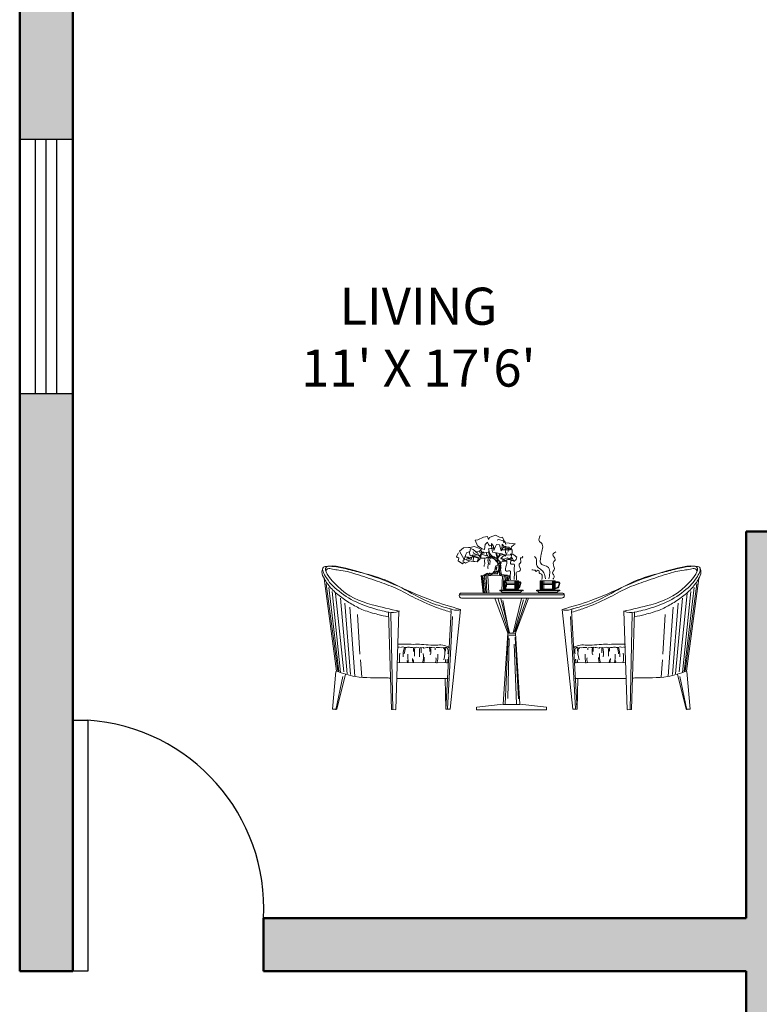
# Model space of a CAD drawing. Units: inches. Extents: x 1771 to 3025, y 319 to 889.
# Tile 2 of 35: x 1800 to 1939, y 527 to 713. Entities that reach past the tile are written whole.
import ezdxf

# ---------------------------------------------------------------- set-up
doc = ezdxf.new("R2010")
doc.units = ezdxf.units.IN
doc.header["$MEASUREMENT"] = 0
for name, color, linetype, lineweight in [('A-AREA-IDEN', 241, 'Continuous', 25), ('A-DOOR', 4, 'Continuous', 25), ('A-FURN', 8, 'Continuous', 18), ('A-GLAZ', 40, 'Continuous', 25), ('A-WALL', 7, 'Continuous', 50), ('A-WALL-PATT', 254, 'Continuous', 13)]:
    doc.layers.add(name, color=color, linetype=linetype, lineweight=lineweight)
doc.styles.get("Standard").update_dxf_attribs({"font": 'arial.ttf'})

# ---------------------------------------------------------------- blocks, each defined once
blk = doc.blocks.new('A$C7D4176DC')
for p, q in [((936.5, 1019.3), (919.6, 1018.3)), ((919.6, 1018.3), (933.7, 984.6)), ((969.3, 1036.1), (936.5, 1019.3)), ((994.5, 1040.8), (969.3, 1036.1)), ((980.5, 991.2), (994.5, 1005.2)), ((1000.2, 1022.1), (994.5, 1040.8)), ((994.5, 1005.2), (999.2, 992.1)), ((1008.6, 1036.1), (1000.2, 1022.1)), ((1010.5, 1037.1), (1041.4, 1048.3)), ((1041.4, 1048.3), (1064.8, 1036.1)), ((1051.7, 1018.3), (1059.2, 1023)), ((1059.2, 1023), (1090.1, 1013.6)), ((1064.8, 1036.1), (1077, 1034.2)), ((1077, 1034.2), (1084.5, 1035.2)), ((1084.5, 1035.2), (1097.6, 1007.1)), ((1091, 1009.9), (1088.2, 1005.2)), ((1088.2, 1005.2), (1104.1, 1009)), ((1090.1, 1013.6), (1091, 1009.9)), ((1104.1, 1009), (1091, 1005.2)), ((1091, 1005.2), (1100.4, 1003.4)), ((850.3, 971.5), (825.9, 951.9)), ((825.9, 951.9), (853.1, 902.3)), ((879.3, 973.4), (850.3, 971.5)), ((869, 944.4), (886.8, 949.1)), ((889.6, 974.3), (879.3, 973.4)), ((890.6, 924.7), (884, 950)), ((886.8, 949.1), (892.4, 968.7)), ((914, 980.9), (889.6, 974.3)), ((892.4, 968.7), (908.4, 962.2)), ((908.4, 962.2), (934.6, 940.6)), ((909.3, 940.6), (908.4, 947.2)), ((947.7, 967.8), (914, 980.9)), ((927.4, 947.9), (955.2, 956.5)), ((933.7, 984.6), (961.8, 966.8)), ((946.8, 953.7), (945.8, 946.2)), ((945.8, 946.2), (971.1, 945.3)), ((958, 965.9), (946.8, 953.7)), ((955.2, 956.5), (961.8, 934.1)), ((961.8, 966.8), (976.7, 961.2)), ((976.7, 961.2), (980.5, 991.2)), ((999.2, 992.1), (1006.7, 983.7)), ((999.2, 965.9), (1016.1, 967.8)), ((1003, 952.8), (999.2, 965.9)), ((999.2, 945.3), (1003, 952.8)), ((1002, 948.1), (1001.1, 940.6)), ((1012.3, 931.3), (1002, 948.1)), ((1006.7, 983.7), (1022.6, 987.4)), ((1022.6, 987.4), (1015.2, 989.3)), ((1016.1, 967.8), (1017, 970.6)), ((1029.2, 982.8), (1017, 998.7)), ((1017, 998.7), (1017, 981.8)), ((1017, 981.8), (1024.5, 946.2)), ((1017, 970.6), (1037.6, 969.7)), ((1024.5, 946.2), (1082.6, 936)), ((1032, 956.5), (1029.2, 982.8)), ((1042.3, 979.9), (1032, 956.5)), ((1037.6, 969.7), (1033, 971.5)), ((1047.9, 992.1), (1042.3, 979.9)), ((1066.7, 989.3), (1047.9, 992.1)), ((1075.1, 953.7), (1066.7, 989.3)), ((1079.8, 959.4), (1075.1, 953.7)), ((1081.7, 994), (1079.8, 959.4)), ((1095.7, 976.2), (1081.7, 994)), ((1103.2, 982.8), (1084.5, 969.7)), ((1084.5, 969.7), (1084.5, 959.4)), ((1084.5, 959.4), (1127.6, 960.3)), ((1121, 975.3), (1095.7, 976.2)), ((1100.4, 1003.4), (1103.2, 993.1)), ((1100.4, 971.5), (1103.2, 982.8)), ((1101.3, 940.6), (1100.4, 971.5)), ((1106, 966.8), (1104.1, 968.7)), ((1121, 969.7), (1106, 966.8)), ((1108.2, 1001.8), (1157.5, 996.8)), ((1119.1, 963.1), (1121, 969.7)), ((1127.6, 960.3), (1119.1, 963.1)), ((1132.2, 960.3), (1121, 975.3)), ((1137.9, 978.1), (1132.2, 960.3)), ((1151, 989.3), (1137.9, 978.1)), ((1159.4, 994), (1151, 989.3)), ((1157.5, 996.8), (1159.4, 994)), ((820.3, 941.6), (808.1, 920)), ((808.1, 920), (811.9, 913.5)), ((811.9, 913.5), (821.2, 911.6)), ((821.2, 911.6), (817.5, 893.8)), ((817.5, 893.8), (843.7, 875.1)), ((847.5, 897.6), (877.4, 906)), ((847.5, 880.7), (847.5, 897.6)), ((853.1, 902.3), (863.4, 931.3)), ((860.6, 917.2), (858.7, 916.3)), ((863.4, 917.2), (860.6, 917.2)), ((878.4, 916.3), (861.5, 919.1)), ((886.7, 892.7), (862.1, 880.4)), ((863.4, 931.3), (869, 944.4)), ((876.5, 911.6), (863.4, 917.2)), ((870.3, 898.8), (868.3, 907)), ((895, 892.7), (870.3, 898.8)), ((879.3, 906.9), (876.5, 911.6)), ((877.4, 906), (884.9, 905.1)), ((883.1, 912.5), (878.4, 916.3)), ((894.3, 912.5), (879.3, 906.9)), ((910.2, 917.2), (883.1, 912.5)), ((884.9, 905.1), (889.6, 903.2)), ((889.6, 903.2), (895.2, 901.3)), ((900.9, 928.5), (890.6, 924.7)), ((902.7, 916.3), (894.3, 912.5)), ((931.9, 888.6), (895, 892.7)), ((895.2, 901.3), (899, 917.2)), ((922.4, 927.5), (900.9, 928.5)), ((903.7, 927.5), (902.7, 916.3)), ((905.6, 928.5), (903.7, 927.5)), ((904.6, 923.8), (905.6, 928.5)), ((904.6, 920), (904.6, 923.8)), ((919.6, 920), (904.6, 920)), ((909.3, 913.2), (907.3, 892.7)), ((917.7, 936), (909.3, 940.6)), ((917.5, 890.6), (909.3, 890.6)), ((939.3, 910.7), (910.2, 917.2)), ((931.9, 888.6), (917.5, 890.6)), ((928, 933.1), (917.7, 936)), ((939.3, 913.5), (919.6, 920)), ((932.7, 929.4), (922.4, 927.5)), ((942.1, 925.7), (928, 933.1)), ((940.1, 909.1), (931.9, 888.6)), ((950.4, 907), (931.9, 888.6)), ((941.1, 929.4), (932.7, 929.4)), ((934.6, 940.6), (938.3, 938.8)), ((985.2, 912.5), (939.3, 910.7)), ((951.5, 911.6), (941.1, 929.4)), ((950.5, 917.2), (942.1, 925.7)), ((955.2, 940.6), (946.8, 924.7)), ((946.8, 924.7), (951.5, 918.2)), ((1026.4, 913.5), (950.4, 907.4)), ((952.4, 910.7), (950.5, 917.2)), ((959.9, 938.8), (951.5, 925.7)), ((951.5, 925.7), (954.3, 912.5)), ((951.5, 918.2), (951.5, 911.6)), ((954.3, 909.7), (955.2, 940.6)), ((954.3, 912.5), (954.3, 909.7)), ((986.1, 943.4), (960.8, 940.6)), ((961.8, 934.1), (984.2, 923.8)), ((967.4, 939.2), (999.2, 945.3)), ((976.2, 896.9), (974.8, 892)), ((974.8, 892), (977.6, 877.4)), ((978.3, 903.2), (976.2, 896.9)), ((977.6, 912.2), (978.3, 903.2)), ((984.2, 923.8), (995.5, 925.7)), ((988.9, 914.4), (985.2, 912.5)), ((989.9, 930.3), (986.1, 943.4)), ((991.7, 916.3), (988.9, 914.4)), ((989.5, 915.7), (998.5, 919.9)), ((995.5, 925.7), (989.9, 930.3)), ((1005.8, 917.2), (991.7, 916.3)), ((998.5, 904.6), (995.7, 898.3)), ((995.7, 898.3), (999.9, 878.8)), ((998.5, 919.9), (1000.6, 912.2)), ((1000.6, 912.2), (998.5, 904.6)), ((1001.1, 940.6), (1006.7, 926.6)), ((1006.9, 906), (1004.1, 898.3)), ((1004.1, 898.3), (1009, 894.8)), ((1007.7, 920), (1005.8, 917.2)), ((1006.7, 926.6), (1011.4, 921.9)), ((1011.8, 911.5), (1006.9, 906)), ((1006.9, 911.5), (1030.6, 908)), ((1009, 889.2), (1006.9, 877.4)), ((1027.3, 916.3), (1007.7, 920)), ((1009, 894.8), (1009, 889.2)), ((1009.7, 920.6), (1011.8, 911.5)), ((1011.4, 921.9), (1025.5, 914.4)), ((1021.7, 921.9), (1012.3, 931.3)), ((1033, 919.1), (1021.7, 921.9)), ((1025.5, 914.4), (1048.9, 908.8)), ((1030.6, 908), (1036.9, 901.1)), ((1046.7, 908.7), (1033, 919.1)), ((1036.9, 901.1), (1049.5, 899)), ((1039, 899), (1045.3, 891.3)), ((1049.5, 899), (1039, 899)), ((1047.9, 941.6), (1043.3, 939.7)), ((1043.3, 939.7), (1048.9, 920)), ((1045.3, 891.3), (1052.3, 886.4)), ((1055.4, 914.4), (1047.9, 941.6)), ((1048.9, 920), (1049.8, 910.7)), ((1048.9, 908.8), (1076, 881.7)), ((1049.8, 910.7), (1050.8, 902.3)), ((1050.8, 902.3), (1060.1, 872.3)), ((1058.2, 880.7), (1050.8, 894.8)), ((1067.6, 934.1), (1054.5, 910.7)), ((1054.5, 910.7), (1054.5, 898.5)), ((1054.5, 898.5), (1059.9, 896.9)), ((1056.4, 890.1), (1055.4, 914.4)), ((1056.4, 905.1), (1055.4, 895.7)), ((1055.4, 895.7), (1057.3, 892)), ((1061.1, 918.2), (1056.4, 905.1)), ((1064.8, 923.8), (1061.1, 918.2)), ((1067.6, 929.4), (1064.8, 927.5)), ((1066.7, 926.6), (1064.8, 923.8)), ((1089.2, 931.3), (1066.7, 926.6)), ((1084.5, 932.2), (1067.6, 929.4)), ((1070.4, 862.9), (1067.6, 890.1)), ((1072.3, 910), (1078.2, 913)), ((1091.3, 904.2), (1072.3, 910)), ((1097.2, 895.4), (1076.7, 886.6)), ((1078.2, 913), (1100.1, 932)), ((1082.6, 936), (1096.7, 928.5)), ((1098.6, 893.9), (1089.9, 904.2)), ((1113.3, 911.5), (1091.3, 904.2)), ((1096.7, 928.5), (1101.3, 922.8)), ((1100.1, 932), (1097.2, 927.6)), ((1097.2, 927.6), (1117.7, 930.5)), ((1113.3, 902.7), (1097.2, 895.4)), ((1113.3, 899.8), (1098.6, 893.9)), ((1101.3, 922.8), (1111.6, 941.6)), ((1111.6, 941.6), (1101.3, 940.6)), ((1122.1, 904.2), (1113.3, 911.5)), ((1127.9, 901.3), (1113.3, 899.8)), ((1117.7, 930.5), (1139.6, 927.6)), ((1138.2, 914.4), (1122.1, 904.2)), ((1138.2, 895.4), (1127.9, 901.3)), ((1129.4, 933.4), (1145.5, 933.4)), ((1144, 908.6), (1138.2, 914.4)), ((1151.3, 895.4), (1138.2, 895.4)), ((1151.3, 891), (1144, 908.6)), ((1145.5, 933.4), (1160.1, 923.2)), ((1166, 901.3), (1151.3, 891)), ((1160.1, 923.2), (1166, 918.8)), ((1166, 918.8), (1170.4, 917.3)), ((1170.4, 917.3), (1166, 901.3)), ((843.7, 875.1), (847.5, 880.7)), ((862.1, 880.4), (853.9, 886.5)), ((977.6, 875.3), (973.4, 867.6)), ((973.4, 867.6), (973.4, 860.6)), ((977.6, 877.4), (977.6, 875.3)), ((997.1, 872.5), (996.4, 855.8)), ((996.4, 855.8), (996.4, 850.9)), ((996.4, 850.9), (997.8, 845.3)), ((999.9, 878.8), (997.1, 872.5)), ((1008.3, 872.5), (1004.8, 871.8)), ((1006.9, 877.4), (1008.3, 872.5)), ((1060.6, 835.8), (1015.2, 815.4)), ((1029.9, 828.6), (1026.5, 819.5)), ((1032, 829.3), (1029.9, 828.6)), ((1033.4, 828.6), (1032, 829.3)), ((1036.9, 832), (1033.4, 828.6)), ((1037.6, 834.1), (1036.9, 832)), ((1044.5, 828.1), (1037.2, 822.3)), ((1039, 850.9), (1037.6, 836.2)), ((1037.6, 836.2), (1037.6, 834.1)), ((1039.7, 853), (1039, 850.9)), ((1044.6, 864.1), (1039.7, 853)), ((1048.9, 832.5), (1044.5, 828.1)), ((1050.9, 864.8), (1044.6, 864.1)), ((1048.1, 856.4), (1045.3, 850.2)), ((1045.3, 850.2), (1045.3, 839)), ((1045.3, 839), (1048.1, 841.1)), ((1048.1, 841.1), (1048.8, 853.7)), ((1048.8, 853.7), (1048.8, 857.1)), ((1057.7, 829.6), (1048.9, 832.5)), ((1049.8, 817.1), (1076, 851.7)), ((1055.8, 873.9), (1050.9, 864.8)), ((1052.3, 886.4), (1057.9, 876.7)), ((1054.7, 813.5), (1057.7, 829.6)), ((1057.9, 876.7), (1055.8, 873.9)), ((1064.4, 865.4), (1056.9, 822.4)), ((1060.1, 872.3), (1058.2, 880.7)), ((1069.5, 859.2), (1059.2, 870.4)), ((1065.7, 884.5), (1061.1, 875.1)), ((1061.1, 875.1), (1061.1, 857.3)), ((1061.1, 857.3), (1064.8, 853.6)), ((1064.8, 853.6), (1069.5, 859.2)), ((1074.2, 859.2), (1065.7, 884.5)), ((1070.4, 864.8), (1065.7, 823.6)), ((1076, 851.7), (1070.4, 864.8)), ((1074.2, 829.2), (1070.4, 862.9)), ((1076, 881.7), (1071.4, 876)), ((1071.4, 876), (1073.2, 863.9)), ((1073.2, 863.9), (1074.2, 859.2)), ((1076.7, 886.6), (1073.8, 883.7)), ((1077, 814.3), (1074.2, 829.2)), ((13.4, 788.5), (86.9, 232)), ((968.4, 700.9), (955.2, 806.2)), ((955.2, 806.2), (1126.5, 803.3)), ((959.3, 806.1), (972.5, 701.9)), ((965.6, 806.1), (976.7, 700.5)), ((976.6, 787.5), (968.6, 786.7)), ((968.6, 786.7), (971.7, 756.8)), ((991.6, 820.2), (969.9, 808.3)), ((975.3, 805.4), (983, 701.2)), ((979.7, 757.6), (976.6, 787.5)), ((979.4, 811.3), (977.9, 801.1)), ((991.8, 816.4), (978.6, 806.2)), ((985.8, 805.4), (990.6, 701.9)), ((1016.7, 816), (991.6, 820.2)), ((1003.5, 807.6), (991.8, 816.4)), ((996.2, 804.1), (1001.1, 701.9)), ((1009.4, 822.3), (1002, 816.4)), ((1002, 816.4), (1054.7, 813.5)), ((1013.7, 810.6), (1003.5, 807.6)), ((1041.6, 819.3), (1013.7, 810.6)), ((1022.3, 819.5), (1016.7, 816)), ((1024.4, 819.5), (1022.3, 819.5)), ((1026.5, 819.5), (1024.4, 819.5)), ((1037.2, 822.3), (1041.6, 819.3)), ((1051.7, 827.4), (1049.8, 817.1)), ((1065.7, 823.6), (1077, 814.3)), ((1066.4, 817.9), (1066.4, 812)), ((1066.4, 812), (1075.2, 806.2)), ((1075.2, 806.2), (1073.8, 812)), ((1073.8, 812), (1114.7, 807.6)), ((1098.2, 804.7), (1077.7, 804.7)), ((1083.8, 803.4), (1080.4, 718.8)), ((1088.8, 774.3), (1088.8, 724.7)), ((1179, 774.3), (1088.8, 774.3)), ((1090.9, 774.1), (1090.9, 725.1)), ((1093.6, 804.7), (1091.9, 774.3)), ((1093.9, 773.8), (1093.9, 725.1)), ((1114.7, 807.6), (1097.2, 801.8)), ((1098.4, 774.1), (1098.4, 724.9)), ((1104, 802), (1101.5, 774.3)), ((1104.1, 773.8), (1104.1, 763.6)), ((1110.9, 799.9), (1108, 774.3)), ((1117.9, 803.4), (1113.7, 774.3)), ((1125, 803.3), (1120, 774.3)), ((1158.2, 773.8), (1158.2, 725.1)), ((1164.1, 773.8), (1164.1, 724.9)), ((1168.6, 774.3), (1168.6, 725.4)), ((1172.9, 774.1), (1172.9, 767.4)), ((1175.9, 774.1), (1175.9, 767.3)), ((1178, 773.8), (1178, 767.2)), ((1179, 767.3), (1179, 774.3)), ((1309.2, 774.3), (1309.2, 724.7)), ((1399.4, 774.3), (1309.2, 774.3)), ((1311, 774.3), (1311, 725)), ((1313.8, 774.6), (1313.8, 724)), ((1318.3, 774.3), (1318.3, 725.2)), ((1324.3, 774.1), (1324.3, 725.5)), ((1331.2, 774.1), (1331.2, 725)), ((1383.9, 774.1), (1383.9, 725.2)), ((1389.2, 774.1), (1389.2, 724.8)), ((1393.7, 774.1), (1393.7, 724.5)), ((1396.6, 774.1), (1396.6, 724.8)), ((1398.3, 774.1), (1398.3, 724.8)), ((1399.4, 724.7), (1399.4, 774.3)), ((2261.7, 788.5), (2188.2, 232)), ((24.7, 755.7), (94.7, 231.2)), ((41.1, 733.1), (100.8, 229.1)), ((61.7, 710.4), (111.1, 223)), ((971.7, 756.8), (979.7, 757.6)), ((1206.9, 718.8), (1068.5, 718.8)), ((1205.1, 715), (1070.7, 715)), ((1100.8, 759), (1088.8, 759)), ((1088.8, 724.7), (1179, 724.7)), ((1100.8, 751.4), (1090.1, 751.4)), ((1093.2, 718.3), (1093.2, 724.5)), ((1100.8, 763.6), (1100.8, 747.6)), ((1107.3, 763.6), (1100.8, 763.6)), ((1100.8, 747.6), (1107.3, 747.6)), ((1101.3, 745), (1101.3, 740.5)), ((1107.3, 745), (1101.3, 745)), ((1101.3, 740.5), (1107.3, 740.5)), ((1104.1, 747.6), (1104.1, 745)), ((1104.1, 740.5), (1104.1, 724.7)), ((1107.3, 747.6), (1107.3, 763.6)), ((1179, 759), (1107.3, 759)), ((1179, 751.4), (1107.3, 751.4)), ((1107.3, 740.5), (1107.3, 745)), ((1172.9, 762.7), (1172.9, 734.9)), ((1172.9, 732.2), (1172.9, 725.1)), ((1173.3, 725.1), (1173.3, 718.3)), ((1175.9, 762.6), (1175.9, 734.6)), ((1175.9, 731.8), (1175.9, 724.6)), ((1178.3, 762.6), (1178.3, 734.8)), ((1178.3, 731.3), (1178.3, 725.1)), ((1179, 734.4), (1179, 762.7)), ((1179, 724.7), (1179, 731.4)), ((1427.3, 718.8), (1288.9, 718.8)), ((1425.4, 715), (1291, 715)), ((1319.1, 759), (1309.2, 759)), ((1309.2, 724.7), (1399.4, 724.7)), ((1319.1, 751.4), (1310.5, 751.4)), ((1313.5, 718.3), (1313.5, 724.5)), ((1319.1, 764.9), (1319.1, 742.2)), ((1323.5, 764.9), (1319.1, 764.9)), ((1319.1, 742.2), (1323.5, 742.2)), ((1319.8, 739.2), (1319.8, 735.6)), ((1322.7, 739.2), (1319.8, 739.2)), ((1319.8, 735.6), (1322.7, 735.6)), ((1322.7, 735.6), (1322.7, 739.2)), ((1323.5, 742.2), (1323.5, 764.9)), ((1399.4, 759), (1323.5, 759)), ((1399.4, 751.4), (1323.5, 751.4)), ((1393.7, 725.1), (1393.7, 718.3)), ((2213.3, 710.4), (2163.9, 223)), ((2233.9, 733.1), (2174.2, 229.1)), ((2250.4, 755.7), (2180.4, 231.2)), ((82.3, 698.1), (131.7, 227.1)), ((111.1, 669.3), (152.3, 214.7)), ((1452.4, 690.9), (826.8, 690.9)), ((1438.5, 700.9), (838.5, 700.9)), ((1438.5, 670.9), (838.5, 670.9)), ((1107.4, 700.9), (968.4, 700.9)), ((1037.2, 670.1), (1115.4, 459.8)), ((1054.9, 670.7), (1122.1, 460.1)), ((1073, 665.2), (1125.7, 463.7)), ((1079.9, 707.4), (1079.6, 701.2)), ((1192.2, 706.1), (1080.1, 706.6)), ((1191.5, 704.8), (1081.7, 704.8)), ((1083.3, 700.5), (1083.3, 704.5)), ((1085.8, 656.2), (1122.1, 471)), ((1198.4, 667), (1147.5, 461.9)), ((1209.3, 659.8), (1156.6, 467.4)), ((1227.5, 665.2), (1160.2, 467.4)), ((1239.7, 670.1), (1161.5, 459.8)), ((1189, 704.5), (1189, 700.5)), ((1412.6, 706.1), (1300.5, 706.6)), ((1411.9, 704.8), (1302.1, 704.8)), ((1303.7, 700.5), (1303.7, 704.5)), ((1409.4, 704.5), (1409.4, 700.5)), ((2163.9, 669.3), (2122.8, 214.7)), ((2192.8, 698.1), (2143.4, 227.1)), ((137.9, 640.5), (170.8, 210.6)), ((166.7, 615.8), (197.6, 202.4)), ((776.4, 594.8), (742.7, 4.4)), ((795.6, 597.2), (767.4, 606)), ((832.5, 602.2), (768.9, 2.8)), ((772.6, 598.5), (776.4, 598.5)), ((825, 598.5), (795.6, 597.2)), ((1442.6, 602.2), (1506.2, 2.8)), ((1450.1, 598.5), (1479.4, 597.2)), ((1479.4, 597.2), (1507.7, 606)), ((1502.4, 598.5), (1498.7, 598.5)), ((1498.7, 594.8), (1532.3, 4.4)), ((2108.4, 615.8), (2077.5, 202.4)), ((2137.2, 640.5), (2104.3, 210.6)), ((214, 572.6), (228.4, 334)), ((398.7, 587.3), (417.4, 0.9)), ((413.7, 579.8), (424.7, 0.9)), ((462.3, 591), (443.8, 0.9)), ((783.9, 560.6), (752.8, 5.4)), ((1491.2, 560.6), (1522.3, 5.4)), ((1812.8, 591), (1831.2, 0.9)), ((1861.4, 579.8), (1850.3, 0.9)), ((1876.4, 587.3), (1857.7, 0.9)), ((2061, 572.6), (2046.6, 334)), ((1115.4, 459.8), (1088.3, 33.1)), ((1118.5, 442), (1100.3, 33.5)), ((1163.9, 447.4), (1114.8, 447.4)), ((1161.5, 459.8), (1115.4, 459.8)), ((1123.9, 427.4), (1116.6, 68)), ((1160.2, 436.5), (1180.2, 66.2)), ((1161.5, 459.8), (1188.6, 33.1)), ((465.7, 375.8), (456.5, 375.8)), ((484.1, 377.3), (471.9, 374.3)), ((499.5, 372.7), (484.1, 377.3)), ((508.7, 374.3), (499.5, 372.7)), ((513.3, 375.8), (508.7, 374.3)), ((525.5, 375.8), (513.3, 375.8)), ((531.7, 374.3), (525.5, 375.8)), ((543.9, 374.3), (531.7, 374.3)), ((547, 371.2), (543.9, 374.3)), ((567, 375.8), (547, 371.2)), ((582.3, 374.3), (567, 375.8)), ((593, 371.2), (590, 374.3)), ((606.8, 372.7), (593, 371.2)), ((611.4, 369.7), (606.8, 372.7)), ((629.8, 372.7), (611.4, 369.7)), ((636, 374.3), (629.8, 372.7)), ((643.6, 375.8), (636, 374.3)), ((648.2, 372.7), (643.6, 375.8)), ((659, 372.7), (648.2, 372.7)), ((677.4, 371.2), (659, 372.7)), ((678.9, 371.2), (678.9, 359)), ((697.3, 374.3), (685.1, 372.7)), ((706.5, 374.3), (697.3, 374.3)), ((715.7, 371.2), (706.5, 374.3)), ((729.5, 372.7), (715.7, 371.2)), ((740.3, 374.3), (729.5, 368.2)), ((729.5, 368.2), (729.5, 372.7)), ((747.9, 374.3), (740.3, 374.3)), ((751, 369.7), (747.9, 374.3)), ((760.2, 374.3), (751, 369.7)), ((1154.8, 393), (1167.5, 35.4)), ((1514.9, 374.3), (1524.1, 369.7)), ((1524.1, 369.7), (1527.1, 374.3)), ((1527.1, 374.3), (1534.8, 374.3)), ((1534.8, 374.3), (1545.5, 368.2)), ((1545.5, 372.7), (1559.3, 371.2)), ((1545.5, 368.2), (1545.5, 372.7)), ((1559.3, 371.2), (1568.5, 374.3)), ((1568.5, 374.3), (1577.7, 374.3)), ((1577.7, 374.3), (1590, 372.7)), ((1596.2, 371.2), (1596.2, 359)), ((1597.7, 371.2), (1616.1, 372.7)), ((1616.1, 372.7), (1626.8, 372.7)), ((1626.8, 372.7), (1631.4, 375.8)), ((1631.4, 375.8), (1639.1, 374.3)), ((1639.1, 374.3), (1645.2, 372.7)), ((1645.2, 372.7), (1663.6, 369.7)), ((1663.6, 369.7), (1668.2, 372.7)), ((1668.2, 372.7), (1682, 371.2)), ((1682, 371.2), (1685.1, 374.3)), ((1692.8, 374.3), (1708.1, 375.8)), ((1708.1, 375.8), (1728.1, 371.2)), ((1728.1, 371.2), (1731.1, 374.3)), ((1731.1, 374.3), (1743.4, 374.3)), ((1743.4, 374.3), (1749.5, 375.8)), ((1749.5, 375.8), (1761.8, 375.8)), ((1761.8, 375.8), (1766.4, 374.3)), ((1766.4, 374.3), (1775.6, 372.7)), ((1775.6, 372.7), (1790.9, 377.3)), ((1790.9, 377.3), (1803.2, 374.3)), ((1809.3, 375.8), (1818.5, 375.8)), ((230.5, 299.1), (238.7, 196.2)), ((2044.6, 299.1), (2036.3, 196.2)), ((756.8, 280.8), (451.1, 284.6)), ((1518.3, 280.8), (1824, 284.6)), ((84, 230.1), (64.2, 2.8)), ((126, 200.5), (84, 0.3)), ((140.9, 212.8), (88.9, 2.8)), ((447.3, 187.5), (757.7, 187.5)), ((739, 187.5), (742.7, 4.4)), ((1827.8, 187.5), (1517.4, 187.5)), ((1536.1, 187.5), (1532.3, 4.4)), ((2134.2, 212.8), (2186.2, 2.8)), ((2149.1, 200.5), (2191.1, 0.3)), ((2191.1, 230.1), (2210.9, 2.8)), ((64.2, 2.8), (88.9, 2.8)), ((417.4, 0.9), (443.8, 0)), ((742.7, 4.4), (746.5, 38)), ((742.7, 4.4), (768.9, 2.8)), ((927.1, 15), (927.1, 0)), ((1088.3, 33.1), (929, 15)), ((1187.5, 31.7), (1087.6, 31.7)), ((1188.6, 33.1), (1348, 15)), ((1348, 15), (1348, 0)), ((1532.3, 4.4), (1506.2, 2.8)), ((1532.3, 4.4), (1528.6, 38)), ((1857.7, 0.9), (1831.3, 0)), ((2210.9, 2.8), (2186.2, 2.8)), ((1348, 0), (927.1, 0))]:
    blk.add_line(p, q)
for centre, radius, start, end in [((1069.4, 716.9), 2.21, 114.75071, 294.8305), ((1059.6, 691.4), 25.9, 31.12717, 65.45392), ((1208.6, 696.5), 19, 99.79621, 154.31096), ((1206.2, 716.7), 1.95, 244.55032, 96.50843), ((1289.8, 716.9), 2.21, 114.75071, 294.8305), ((1280, 691.4), 25.9, 31.12717, 65.45392), ((1429, 696.5), 19, 99.79621, 154.31096), ((1426.6, 716.7), 1.95, 244.55032, 96.50843), ((838.2, 685.9), 15, 89.02539, 270.97461), ((1440.2, 685.9), 15.1, 263.50595, 96.49405), ((421.9, 675.7), 92.7, 253.90068, 295.36386), ((1853.1, 675.7), 92.7, 244.63614, 286.09932), ((631.7, 325.3), 145, 160.46362, 183.26427), ((661.3, 321.8), 167.8, 162.1481, 175.52768), ((592, 359.5), 42.9, 161.29008, 193.50095), ((755.4, 341.1), 200.6, 170.95256, 185.34949), ((841.5, 337.8), 255.8, 172.03905, 184.65389), ((943.9, 345.9), 348.8, 175.42446, 180.75439), ((590.6, 356.2), 56.7, 354.25823, 16.89433), ((579.3, 354.7), 74.8, 340.32989, 13.94105), ((619.9, 341.7), 118.4, 339.52102, 14.35705), ((693.6, 357.6), 48.4, 353.58471, 16.22063), ((689.2, 351.2), 68.2, 347.09902, 16.48344), ((1585.8, 351.2), 68.2, 163.51656, 192.90098), ((1581.5, 357.6), 48.4, 163.77937, 186.41529), ((1655.1, 341.7), 118.4, 165.64295, 200.47898), ((1695.8, 354.7), 74.8, 166.05895, 199.67011), ((1684.4, 356.2), 56.7, 163.10567, 185.74177), ((1331.2, 345.9), 348.8, 359.24561, 4.57554), ((1433.6, 337.8), 255.8, 355.34611, 7.96095), ((1519.7, 341.1), 200.6, 354.65051, 9.04744), ((1683.1, 359.5), 42.9, 346.49905, 18.70992), ((1613.7, 321.8), 167.8, 4.47232, 17.8519), ((1643.3, 325.3), 145, 356.73573, 19.53638), ((665.2, 310.8), 200.4, 171.53233, 187.34342), ((522.1, 292), 10.6, 155.04372, 216.38582), ((746.2, 323.3), 231.2, 177.65923, 189.89094), ((596.6, 305.3), 53.4, 177.23164, 203.39317), ((-475.8, 101.1), 1042.4, 10.14258, 11.10952), ((484.6, 319.5), 124.8, 342.71731, 8.30681), ((204.5, 341.5), 411.6, 351.83053, 356.14259), ((645.6, 301.5), 39.5, 333.88539, 14.90767), ((494.8, 326.9), 201, 346.57929, 1.64099), ((682.4, 301.4), 59.8, 341.0378, 359.49279), ((616.9, 303.9), 135.6, 349.74606, 359.61704), ((1658.2, 303.9), 135.6, 180.38296, 190.25394), ((1592.7, 301.4), 59.8, 180.50721, 198.9622), ((1780.3, 326.9), 201, 178.35901, 193.42071), ((1629.4, 301.5), 39.5, 165.09233, 206.11461), ((2070.6, 341.5), 411.6, 183.85741, 188.16947), ((1790.4, 319.5), 124.8, 171.69319, 197.28269), ((2750.9, 101.1), 1042.4, 168.89048, 169.85742), ((1678.5, 305.3), 53.4, 336.60683, 2.76836), ((1528.9, 323.3), 231.2, 350.10906, 2.34077), ((1753, 292), 10.6, 323.61418, 24.95628), ((1609.9, 310.8), 200.4, 352.65658, 8.46767)]:
    blk.add_arc(centre, radius, start, end)
for points, knots in [([(1361.4, 785.9), (1364, 797.1), (1369.1, 819), (1366.1, 867.4), (1305.9, 865.7), (1312.3, 906.5), (1315.7, 942.7), (1336.1, 991.6), (1296, 1015.4), (1304.6, 1034), (1310, 1045.7)], [0, 0, 0, 0, 35.255511, 69.327341, 124.802742, 145.944632, 176.486081, 244.459642, 263.687549, 295.971636, 295.971636, 295.971636, 295.971636]), ([(1154.2, 782.2), (1154.8, 800.5), (1155.7, 825.5), (1152.5, 852.8), (1161, 880.4), (1126, 866.1), (1137.2, 896.5), (1131.8, 923.4), (1156.8, 968.1), (1113.4, 971.1), (1116.9, 957), (1118.7, 949.8)], [0, 0, 0, 0, 53.324624, 72.369114, 91.413604, 110.471764, 134.594802, 149.830446, 204.42477, 220.941926, 238.716972, 238.716972, 238.716972, 238.716972]), ([(1385.6, 784.4), (1390.4, 789.9), (1401.4, 802.3), (1375.2, 822.1), (1401.7, 842.3), (1389.4, 864.6), (1386.5, 887), (1411.5, 904.8), (1373.5, 930.7), (1394.6, 942.4), (1403.7, 947.5)], [0, 0, 0, 0, 18.925439, 42.566292, 64.867201, 90.936936, 109.058775, 128.752565, 161.181972, 185.77482, 185.77482, 185.77482, 185.77482]), ([(1131.4, 779.6), (1130.3, 791.6), (1128.8, 807.5), (1135.2, 839.3), (1091.9, 821.5), (1105.3, 863.2), (1115.5, 900.9), (1079.7, 883.7), (1089.8, 909.5), (1078.6, 906.7), (1072.9, 905.3)], [0, 0, 0, 0, 39.358681, 52.054923, 76.195091, 115.553772, 137.137409, 158.736993, 171.43349, 184.13893, 184.13893, 184.13893, 184.13893]), ([(1166.9, 779.6), (1167.6, 787.2), (1168.9, 801.7), (1159.5, 831.3), (1208.7, 829.6), (1171.7, 871.4), (1202, 885.9), (1182.6, 918), (1207, 909.8), (1204.8, 918.7), (1203.8, 923.1)], [0, 0, 0, 0, 24.123038, 45.706674, 71.213394, 110.655389, 125.899008, 152.561192, 162.725628, 172.882723, 172.882723, 172.882723, 172.882723]), ([(1341.7, 785.9), (1340.2, 798.9), (1337.5, 822.1), (1313, 843.2), (1292.5, 855.8), (1286.2, 880.3), (1292.2, 903.3), (1280.3, 916.5), (1276.7, 920.3)], [0, 0, 0, 0, 37.360481, 67.270583, 93.998428, 104.993238, 141.362472, 156.467713, 156.467713, 156.467713, 156.467713]), ([(398, 584.9), (364.8, 593.1), (288.2, 612.1), (173, 656.7), (78.3, 727.2), (27.8, 785.3), (-11.1, 856.8), (24.4, 860.7), (34.5, 861.8)], [0, 0, 0, 0, 102.450812, 236.341037, 372.740804, 434.264952, 500.538568, 526.867635, 526.867635, 526.867635, 526.867635]), ([(397.9, 557.5), (377.2, 562.2), (327.1, 573.6), (252, 594.7), (177.4, 633.5), (110.3, 676.9), (52.9, 727.5), (17.7, 778.4), (-3, 818.5), (1.2, 838.8), (2.4, 844.5)], [0, 0, 0, 0, 63.757158, 154.207673, 233.111021, 314.773872, 393.990027, 459.45949, 503.309158, 520.507412, 520.507412, 520.507412, 520.507412]), ([(832.5, 602.2), (773.3, 619.4), (552.4, 683.6), (381.9, 796.6), (-38, 894.8), (125.3, 689.4), (274.3, 633.7), (409.7, 603.5), (466, 591)], [0, 0, 0, 0, 179.241333, 669.878405, 853.517726, 978.360591, 1217.111989, 1387.04363, 1387.04363, 1387.04363, 1387.04363]), ([(774.4, 584.9), (749.6, 592.8), (676.5, 616.3), (565.4, 663.8), (449, 732.3), (326.3, 773), (214.5, 813.5), (122.5, 837.9), (67.5, 840.8), (36.8, 851.9), (27.3, 839.8), (24.3, 836)], [0, 0, 0, 0, 78.234212, 230.212389, 361.399227, 482.184421, 615.817971, 721.353317, 759.79292, 789.08251, 802.845503, 802.845503, 802.845503, 802.845503]), ([(778, 604.3), (747.1, 612.4), (671.2, 632.3), (544.7, 691), (406.7, 777.8), (262.4, 816.3), (152.4, 843.8), (83.7, 860.5), (45.9, 861.5), (34.5, 861.8)], [0, 0, 0, 0, 95.639299, 234.867324, 416.660896, 581.537135, 678.863317, 758.06805, 792.133261, 792.133261, 792.133261, 792.133261]), ([(1319.1, 782.9), (1321.9, 795.4), (1325.6, 812.1), (1309.5, 816.4), (1302.3, 822.2), (1305.8, 830.8), (1295.5, 845.6), (1286, 822.9), (1281.2, 839.2), (1270.5, 838.4), (1264.1, 839.6), (1260.1, 840.3)], [0, 0, 0, 0, 30.24085, 40.376736, 46.786017, 54.336911, 66.135106, 80.063877, 89.736225, 97.441532, 109.625491, 109.625491, 109.625491, 109.625491]), ([(1442.6, 602.2), (1501.7, 619.4), (1722.7, 683.6), (1893.2, 796.6), (2313.1, 894.8), (2149.7, 689.4), (2000.7, 633.7), (1865.4, 603.5), (1809.1, 591)], [0, 0, 0, 0, 179.241333, 669.878405, 853.517726, 978.360591, 1217.111989, 1387.04363, 1387.04363, 1387.04363, 1387.04363]), ([(1497.1, 604.3), (1528, 612.4), (1603.8, 632.3), (1730.4, 691), (1868.3, 777.8), (2012.7, 816.3), (2122.7, 843.8), (2191.4, 860.5), (2229.2, 861.5), (2240.6, 861.8)], [0, 0, 0, 0, 95.639299, 234.867324, 416.660896, 581.537135, 678.863317, 758.06805, 792.133261, 792.133261, 792.133261, 792.133261]), ([(1500.6, 584.9), (1525.5, 592.8), (1598.5, 616.3), (1709.7, 663.8), (1826.1, 732.3), (1948.7, 773), (2060.6, 813.5), (2152.5, 837.9), (2207.6, 840.8), (2238.3, 851.9), (2247.7, 839.8), (2250.7, 836)], [0, 0, 0, 0, 78.234212, 230.212389, 361.399227, 482.184421, 615.817971, 721.353317, 759.79292, 789.08251, 802.845503, 802.845503, 802.845503, 802.845503]), ([(1877.1, 584.9), (1910.3, 593.1), (1986.9, 612.1), (2102.1, 656.7), (2196.8, 727.2), (2247.3, 785.3), (2286.2, 856.8), (2250.7, 860.7), (2240.6, 861.8)], [0, 0, 0, 0, 102.450812, 236.341037, 372.740804, 434.264952, 500.538568, 526.867635, 526.867635, 526.867635, 526.867635]), ([(1877.1, 557.5), (1897.9, 562.2), (1947.9, 573.6), (2023.1, 594.7), (2097.7, 633.5), (2164.7, 676.9), (2222.2, 727.5), (2257.3, 778.4), (2278.1, 818.5), (2273.8, 838.8), (2272.7, 844.5)], [0, 0, 0, 0, 63.757158, 154.207673, 233.111021, 314.773872, 393.990027, 459.45949, 503.309158, 520.507412, 520.507412, 520.507412, 520.507412]), ([(1399.4, 767.3), (1402.9, 767.5), (1411.4, 768.1), (1432.6, 770.2), (1424.9, 746.9), (1419.3, 731), (1409, 728.9), (1399.9, 726.6), (1399.4, 728.7), (1399.4, 728.8)], [0, 0, 0, 0, 11.082717, 27.168464, 47.8303, 63.341794, 75.5235, 81.952599, 82.221535, 82.221535, 82.221535, 82.221535]), ([(1169.5, 767.6), (1169.1, 766.9), (1168.6, 765.8), (1168.5, 764.1), (1168.9, 763.4), (1169.1, 763)], [0, 0, 0, 0, 2.454471, 3.694729, 4.863756, 4.863756, 4.863756, 4.863756]), ([(1169.1, 763), (1172.8, 762.7), (1177.7, 762.3), (1183.6, 763.4), (1189.9, 762.9), (1187.4, 754.3), (1187.2, 747.1), (1184.4, 741.1), (1183.6, 734.2), (1179.1, 734.3), (1176.3, 734.5), (1173.7, 734.9), (1171.6, 734.9), (1169.1, 736.3), (1168.8, 734.4), (1168.7, 733.5), (1168.7, 732.9), (1169, 732.2), (1169.6, 732.2), (1169.9, 732.3)], [0, 0, 0, 0, 11.017731, 14.368752, 18.607743, 26.502791, 33.640107, 41.65747, 47.330925, 50.070533, 53.653147, 56.161165, 57.765785, 60.50412, 61.601302, 62.440841, 63.254964, 63.604793, 64.589255, 64.589255, 64.589255, 64.589255]), ([(1169.5, 767.6), (1173.2, 767.4), (1179.9, 766.9), (1197.8, 769.9), (1190.9, 747.3), (1187.7, 728.5), (1175.3, 732.4), (1169.7, 732.3), (1169.1, 732.2)], [0, 0, 0, 0, 11.640419, 20.980802, 45.0396, 57.043585, 71.929427, 73.92866, 73.92866, 73.92866, 73.92866]), ([(1180.5, 766.4), (1182.7, 766.7), (1186, 767.2), (1193.4, 764.4), (1189.7, 753.8), (1188.7, 747.3), (1188.2, 744.3)], [0, 0, 0, 0, 6.446326, 10.075492, 21.292554, 31.027811, 31.027811, 31.027811, 31.027811]), ([(1399.4, 760.8), (1402.3, 761.2), (1409.4, 762.1), (1423.2, 766.3), (1423.3, 753.9), (1420.3, 746.4), (1417.8, 735.7), (1409.3, 733.5), (1403.3, 729.7), (1400.4, 731.6), (1399.4, 732.3)], [0, 0, 0, 0, 9.652474, 22.996839, 29.518582, 40.146055, 49.702279, 58.739504, 65.130432, 68.539734, 68.539734, 68.539734, 68.539734]), ([(763.3, 374.3), (771.1, 374), (721.2, 391.5), (701, 387.4), (647.2, 387.1), (600.7, 394.2), (547.4, 391.8), (499.5, 394.7), (467.3, 394.3), (453.5, 394.2)], [0, 0, 0, 0, 23.359127, 69.600901, 112.546095, 167.952511, 215.499051, 270.735631, 312.147322, 312.147322, 312.147322, 312.147322]), ([(1511.8, 374.3), (1504, 374), (1553.9, 391.5), (1574.1, 387.4), (1627.8, 387.1), (1674.4, 394.2), (1727.7, 391.8), (1775.6, 394.7), (1807.8, 394.3), (1821.6, 394.2)], [0, 0, 0, 0, 23.359127, 69.600901, 112.546095, 167.952511, 215.499051, 270.735631, 312.147322, 312.147322, 312.147322, 312.147322]), ([(86.9, 232), (124.5, 219.1), (220.3, 186.2), (332, 194.5), (402.2, 190.3), (411.4, 189.7)], [0, 0, 0, 0, 118.259021, 301.591906, 329.266035, 329.266035, 329.266035, 329.266035]), ([(2188.2, 232), (2150.6, 219.1), (2054.8, 186.2), (1943.1, 194.5), (1872.9, 190.3), (1863.7, 189.7)], [0, 0, 0, 0, 118.259021, 301.591906, 329.266035, 329.266035, 329.266035, 329.266035])]:
    blk.add_open_spline(points, degree=3, knots=knots)
blk = doc.blocks.new('DOOR-36A')
blk.add_lwpolyline([(0, 47.37), (2.84, 47.37), (2.84, 0), (0, 0)], close=True)
blk.add_arc((0.47, 11.87), 35.58, 356.991, 86.1899)
blk = doc.blocks.new('WIN-48')
for p, q in [((0, 0), (0, 10)), ((48, 0), (48, 10)), ((0, 7), (48, 7)), ((0, 5), (48, 5)), ((0, 3), (48, 3))]:
    blk.add_line(p, q)

msp = doc.modelspace()

# ---------------------------------------------------------------- hatches: boundary and pattern name
at = {"layer": 'A-WALL-PATT'}
h = msp.add_hatch(color=256, dxfattribs=at)
h.dxf.hatch_style = 1
h.paths.add_polyline_path([(1870.72, 888.63), (1799.72, 888.63), (1799.72, 878.63), (1870.72, 878.63)])
h.paths.add_polyline_path([(1968.77, 888.63), (1918.72, 888.63), (1918.72, 878.63), (1941.72, 878.63), (1941.72, 830.63), (1946.72, 830.63), (1946.72, 878.63), (1968.77, 878.63)])
h.paths.add_polyline_path([(2059.68, 888.63), (2016.77, 888.63), (2016.77, 878.63), (2037.72, 878.63), (2037.72, 794.63), (1941.72, 794.63), (1941.72, 758.63), (1941.72, 664.63), (1946.72, 664.63), (1946.72, 712), (1946.72, 789.63), (2054.72, 789.63), (2054.72, 794.63), (2042.33, 794.63), (2042.33, 798.62), (2042.33, 835.5), (2042.72, 878.63), (2059.68, 878.63)])
h.paths.add_polyline_path([(2100.72, 888.63), (2077.68, 888.63), (2077.68, 878.63), (2090.72, 878.63), (2090.72, 789.63), (2090.72, 768.61), (2100.72, 768.61)])
h.paths.add_polyline_path([(2100.72, 720.61), (2090.72, 720.61), (2090.72, 669.63), (1982.72, 669.63), (1982.72, 664.63), (2001.72, 664.63), (2001.72, 652.63), (2006.72, 652.63), (2006.72, 664.63), (2049.52, 664.63, -0.385549), (2050.52, 664.63), (2090.72, 664.63), (2090.72, 649.17), (2100.72, 649.17)])
edge = h.paths.add_edge_path()
edge.add_line((2100.72, 631.17), (2090.72, 631.17))
edge.add_line((2090.72, 631.17), (2090.72, 616.63))
edge.add_line((2090.72, 616.63), (2001.72, 616.63))
edge.add_line((2001.72, 616.63), (1982.72, 616.63))
edge.add_line((1982.72, 616.63), (1982.72, 611.63))
edge.add_line((1982.72, 611.63), (2024.67, 611.63))
edge.add_spline(control_points=[(2024.67, 611.63), (2027.58, 612.87), (2030.01, 613.31), (2032.47, 613.72)], knot_values=[484.321569, 484.321569, 484.321569, 484.321569, 625.498764, 625.498764, 625.498764, 625.498764], degree=3, periodic=0)
edge.add_line((2032.47, 613.72), (2033.2, 613.72))
edge.add_spline(control_points=[(2033.2, 613.72), (2035.66, 613.31), (2039.46, 612.87), (2042.2, 611.63)], knot_values=[484.321569, 484.321569, 484.321569, 484.321569, 625.498764, 625.498764, 625.498764, 625.498764], degree=3, periodic=0)
edge.add_line((2042.2, 611.63), (2090.72, 611.63))
edge.add_line((2090.72, 611.63), (2090.72, 581.11))
edge.add_line((2090.72, 581.11), (2100.72, 581.11))
edge.add_line((2100.72, 581.11), (2100.72, 631.17))
h.paths.add_polyline_path([(2100.72, 533.11), (2090.72, 533.11), (2090.72, 479.63), (1946.72, 479.63), (1946.72, 616.63), (1936.72, 616.63), (1936.72, 543.63), (1845.72, 543.63), (1845.72, 533.63), (1936.72, 533.63), (1936.72, 469.63), (2090.72, 469.63), (2090.72, 452.76), (2100.72, 452.76)])
h.paths.add_polyline_path([(2100.72, 404.76), (2090.72, 404.76), (2090.72, 393.63), (1936.72, 393.63), (1936.72, 383.63), (2100.72, 383.63)])
h.paths.add_polyline_path([(1905.72, 758.63), (1835.47, 758.63), (1835.47, 758.63), (1813.44, 758.63), (1809.72, 758.63), (1809.72, 842.59, -0.008336), (1808.42, 842.63), (1799.72, 842.63), (1799.72, 690.58), (1809.72, 690.58), (1809.72, 753.63), (1905.72, 753.63)])
h.paths.add_polyline_path([(1809.72, 642.58), (1799.72, 642.58), (1799.72, 533.63), (1809.72, 533.63), (1809.72, 581)])

# ---------------------------------------------------------------- linework, layer by layer
at = {"layer": 'A-WALL'}
for p, q in [((1799.72, 842.63), (1799.72, 533.63)), ((1809.72, 753.63), (1809.72, 533.63)), ((1936.72, 616.63), (1936.72, 543.63)), ((1946.72, 616.63), (1936.72, 616.63)), ((1936.72, 543.63), (1845.72, 543.63)), ((1845.72, 543.63), (1845.72, 533.63)), ((1809.72, 533.63), (1799.72, 533.63)), ((1936.72, 533.63), (1845.72, 533.63)), ((1936.72, 533.63), (1936.72, 469.63))]:
    msp.add_line(p, q, dxfattribs=at)

# ---------------------------------------------------------------- block references
at = {"layer": 'A-DOOR'}
msp.add_blockref('DOOR-36A', (1809.72, 533.63), dxfattribs=at)
at = {"layer": 'A-FURN', "xscale": 0.0314240770509951, "yscale": 0.0314240770509951, "zscale": 0.0314240770509951}
msp.add_blockref('A$C7D4176DC', (1856.73, 582.99), dxfattribs=at)
at = {"layer": 'A-GLAZ', "rotation": 90.00000000000124}
msp.add_blockref('WIN-48', (1809.72, 642.58), dxfattribs=at)

# ---------------------------------------------------------------- texts
at = {"layer": 'A-AREA-IDEN', "insert": (1832.19, 662.63), "char_height": 7, "attachment_point": 1}
msp.add_mtext_dynamic_manual_height_columns("\\pxqc;LIVING \\P11' X 17'6'", width=85.4611, gutter_width=1, heights=[0], dxfattribs=at)

doc.saveas('drawing.dxf')
